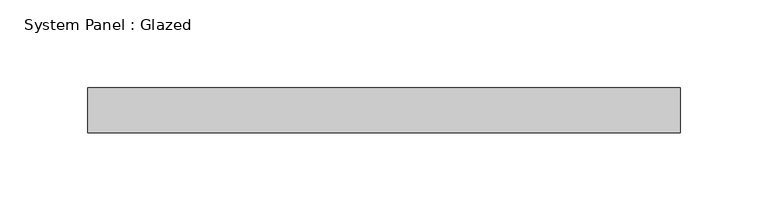
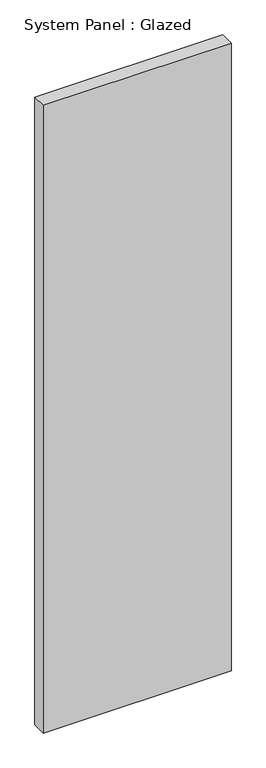
"""IFC4 building model written with IfcOpenShell, lengths in millimetres: plate geometry, System Panel : Glazed."""

from ifc_helpers import new_model, si_unit, origin, origin_with_axes, place, context, project, spatial, polyline, outline, extrude, source, transform, mapped, element, save


def system_panel_glazed_f010d5cf(model_context):
    return source(origin(), model_context, "Body", "SweptSolid", [
        extrude(outline(polyline([(168.275, 19.05), (-168.275, 19.05), (-168.275, 44.45), (168.275, 44.45), (168.275, 19.05)])), origin_with_axes(), (0.0, 0.0, 1.0), 1188.425758),
    ])


if __name__ == "__main__":
    model = new_model("IFC4")
    model_context = context("Model", 3, world=origin())
    ifc_project = project(units=[si_unit("LENGTHUNIT", "METRE", prefix="MILLI")], contexts=[model_context])
    site = spatial("IfcSite", under=ifc_project)
    building = spatial("IfcBuilding", under=site)
    placement = place(None, origin())
    system_panel_glazed_shape = system_panel_glazed_f010d5cf(model_context)
    element("IfcPlate", 1, ObjectType="System Panel : Glazed", at=placement, inside=building, context=model_context, shape_type="MappedRepresentation", body=[
        mapped(system_panel_glazed_shape, transform((0.0, 0.0, 0.0), x_axis=(1.0, 0.0, 0.0), y_axis=(0.0, 1.0, 0.0), z_axis=(0.0, 0.0, 1.0))),
    ])
    save(model, "model.ifc")

# Revit data of these elements
# Type "System Panel : Glazed"
#   Construction Type Id = "GSP4R"
#   Analytic Construction = "1/8 in Pilkington single glazing"
#   Visual Light Transmittance = 0.9
#   Solar Heat Gain Coefficient = 0.86
#   Heat Transfer Coefficient (U) = 1.18115 BTU/(h·ft²·°F)
#   Define Thermal Properties by = 1
# Element 1 (IfcPlate, "System Panel : Glazed")
#   Materials on its faces: "Glass"
# Materials
#   "Glass": class "Glass", colour RGB 0 128 192, transparency 0.75, Description = "Soda Lime Glass", Cost = 0
